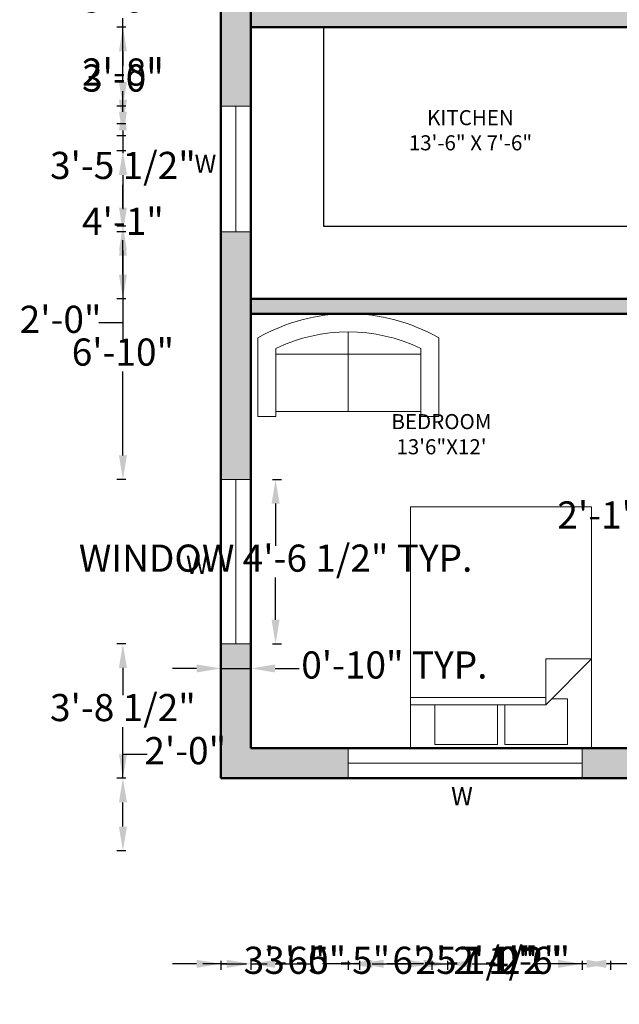
# Model space of a CAD drawing. Units: inches. Extents: x 2568 to 3190, y 746 to 1467.
# Tile 1 of 7: x 2568 to 2767, y 746 to 1073. Entities that reach past the tile are written whole.
import ezdxf

# ---------------------------------------------------------------- set-up
doc = ezdxf.new("R2010")
doc.units = ezdxf.units.IN
for name, color, linetype, lineweight in [('A-ANNO-DIMS', 2, 'Continuous', 18), ('A-ANNO-TEXT', 7, 'Continuous', 18), ('A-AREA-IDEN', 7, 'Continuous', 25), ('A-FLOR-CASE', 8, 'Continuous', 25), ('A-FURN', 8, 'Continuous', 18), ('A-GLAZ', 4, 'Continuous', 20), ('A-WALL', 7, 'Continuous', 50), ('A-WALL-PATT', 252, 'Continuous', 13)]:
    doc.layers.add(name, color=color, linetype=linetype, lineweight=lineweight)
doc.styles.get("Standard").update_dxf_attribs({"font": 'arial.ttf'})
doc.dimstyles.new('ISO-25', dxfattribs={"dimtxt": 9, "dimasz": 8, "dimexe": 2, "dimexo": 1, "dimtad": 0, "dimtih": 1, "dimtoh": 1, "dimdec": 1, "dimlunit": 3, "dimtxsty": 'Standard', "dimcen": 2.5, "dimclrd": 1, "dimclre": 3, "dimclrt": 6, "dimadec": 0, "dimazin": 0, "dimtfac": 1, "dimtdec": 1, "dimtmove": 0, "dimatfit": 3, "dimfxl": 1, "dimfxlon": 1, "dimarcsym": 0})

# ---------------------------------------------------------------- blocks, each defined once
blk = doc.blocks.new('Bed - Queen')
for p, q in [((0, -80.00003), (0, 0)), ((0, 0), (59.99999, 0)), ((59.99999, 0), (59.99999, -80.00003)), ((7.99999, -1.2), (28.79998, -1.2)), ((7.99999, -14.4), (7.99999, -1.2)), ((28.79998, -1.2), (28.79998, -14.4)), ((31.19999, -1.2), (51.99999, -1.2)), ((31.19999, -14.4), (31.19999, -1.2)), ((51.99999, -1.2), (51.99999, -16.4)), ((0, -14.4), (44.8, -14.4)), ((59.99999, -29.6), (44.8, -14.4)), ((44.8, -14.4), (44.8, -29.6)), ((44.8, -16.8), (0, -16.8)), ((51.99999, -16.4), (46.79936, -16.4)), ((44.8, -29.6), (59.99999, -29.6)), ((59.99999, -80.00003), (0, -80.00003))]:
    blk.add_line(p, q)
blk = doc.blocks.new('Sofa - Roundback Loveseat 5 ft.')
for p, q in [((0, -32.44198), (0, -5.99998)), ((-24, -33.99998), (-24, -11.46958)), ((24.00004, -33.99998), (24.00004, -11.46958)), ((-23.9998, -13.38178), (23.99986, -13.38178)), ((-24, -32.44198), (24.00004, -32.44198))]:
    blk.add_line(p, q)
for points in [[(-24, -33.99998), (-30, -33.99998), (-30, -7.99998)], [(30.00004, -7.99998), (30.00004, -33.99998), (24.00004, -33.99998)]]:
    blk.add_lwpolyline(points)
for centre, radius, start, end in [((0, -60.24998), 60.24998, 60.13715, 119.8628), ((0, -61.38438), 55.38444, 64.32083, 115.6792)]:
    blk.add_arc(centre, radius, start, end)
blk = doc.blocks.new('WIN-BED-LOWER-54.48')
for p, q in [((-5, 54.48), (5, 54.48)), ((0, 0), (0, 54.48)), ((5, 0), (-5, 0))]:
    blk.add_line(p, q)
blk = doc.blocks.new('*D26')
at = {"layer": 'A-ANNO-DIMS', "color": 1, "lineweight": -2, "transparency": 16777216}
for p, q in [((2809.71, 907.49), (2801.71, 907.49)), ((2826.58, 907.49), (2817.71, 907.49))]:
    blk.add_line(p, q, dxfattribs=at)
at = {"layer": 'A-ANNO-DIMS', "color": 3, "lineweight": -2, "transparency": 16777216}
for p, q in [((2809.71, 906.49), (2809.71, 909.49)), ((2834.58, 906.49), (2834.58, 909.49))]:
    blk.add_line(p, q, dxfattribs=at)
at = {"layer": 'A-ANNO-DIMS', "color": 1, "transparency": 16777216}
for points in [[(2817.71, 908.82), (2817.71, 906.15), (2809.71, 907.49)], [(2826.58, 908.82), (2826.58, 906.15), (2834.58, 907.49)]]:
    blk.add_solid(points, dxfattribs=at)
at = {"layer": 'Defpoints', "color": 0, "transparency": 16777216}
for p in [(2809.71, 907.49), (2809.71, 898.94), (2834.58, 898.94)]:
    blk.add_point(p, dxfattribs=at)
at = {"layer": 'A-ANNO-DIMS', "color": 6, "transparency": 16777216, "insert": (2773.58, 907.49), "char_height": 9, "attachment_point": 5}
blk.add_mtext('2\'-1" TYP.', dxfattribs=at)
blk = doc.blocks.new('*D35')
at = {"layer": 'A-ANNO-DIMS', "color": 3, "lineweight": -2, "transparency": 16777216}
for p, q in [((2651.69, 920.42), (2654.69, 920.42)), ((2651.69, 865.93), (2654.69, 865.93))]:
    blk.add_line(p, q, dxfattribs=at)
at = {"layer": 'A-ANNO-DIMS', "color": 1, "lineweight": -2, "transparency": 16777216}
for p, q in [((2652.69, 912.42), (2652.69, 898.46)), ((2652.69, 873.93), (2652.69, 887.89))]:
    blk.add_line(p, q, dxfattribs=at)
at = {"layer": 'A-ANNO-DIMS', "color": 1, "transparency": 16777216}
for points in [[(2651.36, 912.42), (2654.03, 912.42), (2652.69, 920.42)], [(2651.36, 873.93), (2654.03, 873.93), (2652.69, 865.93)]]:
    blk.add_solid(points, dxfattribs=at)
at = {"layer": 'Defpoints', "color": 0, "transparency": 16777216}
for p in [(2644.52, 920.42), (2652.69, 920.42), (2644.52, 865.93)]:
    blk.add_point(p, dxfattribs=at)
at = {"layer": 'A-ANNO-DIMS', "color": 6, "transparency": 16777216, "insert": (2652.69, 893.17), "char_height": 9, "attachment_point": 5}
blk.add_mtext('WINDOW 4\'-6 1/2" TYP.', dxfattribs=at)
blk = doc.blocks.new('*D36')
at = {"layer": 'A-ANNO-DIMS', "color": 3, "lineweight": -2, "transparency": 16777216}
for p, q in [((2634.52, 858.76), (2634.52, 855.76)), ((2644.52, 858.76), (2644.52, 855.76))]:
    blk.add_line(p, q, dxfattribs=at)
at = {"layer": 'A-ANNO-DIMS', "color": 1, "lineweight": -2, "transparency": 16777216}
for p, q in [((2626.52, 857.76), (2618.52, 857.76)), ((2634.52, 857.76), (2644.52, 857.76)), ((2652.52, 857.76), (2660.52, 857.76))]:
    blk.add_line(p, q, dxfattribs=at)
at = {"layer": 'A-ANNO-DIMS', "color": 1, "transparency": 16777216}
for points in [[(2626.52, 859.1), (2626.52, 856.43), (2634.52, 857.76)], [(2652.52, 859.1), (2652.52, 856.43), (2644.52, 857.76)]]:
    blk.add_solid(points, dxfattribs=at)
at = {"layer": 'Defpoints', "color": 0, "transparency": 16777216}
for p in [(2634.52, 865.93), (2644.52, 865.93), (2644.52, 857.76)]:
    blk.add_point(p, dxfattribs=at)
at = {"layer": 'A-ANNO-DIMS', "color": 6, "transparency": 16777216, "insert": (2692.07, 857.76), "char_height": 9, "attachment_point": 5}
blk.add_mtext('0\'-10" TYP.', dxfattribs=at)
blk = doc.blocks.new('*D39')
at = {"layer": 'A-ANNO-DIMS', "color": 3, "lineweight": -2, "transparency": 16777216}
for p, q in [((2644.52, 760.85), (2644.52, 757.85)), ((2709.74, 760.85), (2709.74, 757.85))]:
    blk.add_line(p, q, dxfattribs=at)
at = {"layer": 'A-ANNO-DIMS', "color": 1, "lineweight": -2, "transparency": 16777216}
for p, q in [((2652.52, 759.85), (2664.54, 759.85)), ((2701.74, 759.85), (2689.72, 759.85))]:
    blk.add_line(p, q, dxfattribs=at)
at = {"layer": 'A-ANNO-DIMS', "color": 1, "transparency": 16777216}
for points in [[(2652.52, 761.18), (2652.52, 758.51), (2644.52, 759.85)], [(2701.74, 761.18), (2701.74, 758.51), (2709.74, 759.85)]]:
    blk.add_solid(points, dxfattribs=at)
at = {"layer": 'Defpoints', "color": 0, "transparency": 16777216}
for p in [(2644.52, 1411.35), (2709.74, 1411.35), (2709.74, 759.85)]:
    blk.add_point(p, dxfattribs=at)
at = {"layer": 'A-ANNO-DIMS', "color": 6, "transparency": 16777216, "insert": (2677.13, 759.85), "char_height": 9, "attachment_point": 5}
blk.add_mtext('5\'-5"', dxfattribs=at)
blk = doc.blocks.new('*D40')
at = {"layer": 'A-ANNO-DIMS', "color": 3, "lineweight": -2, "transparency": 16777216}
for p, q in [((2709.74, 760.85), (2709.74, 757.85)), ((2763.78, 760.85), (2763.78, 757.85))]:
    blk.add_line(p, q, dxfattribs=at)
at = {"layer": 'A-ANNO-DIMS', "color": 1, "lineweight": -2, "transparency": 16777216}
for p, q in [((2717.74, 759.85), (2723.99, 759.85)), ((2755.78, 759.85), (2749.52, 759.85))]:
    blk.add_line(p, q, dxfattribs=at)
at = {"layer": 'A-ANNO-DIMS', "color": 1, "transparency": 16777216}
for points in [[(2717.74, 761.18), (2717.74, 758.51), (2709.74, 759.85)], [(2755.78, 761.18), (2755.78, 758.51), (2763.78, 759.85)]]:
    blk.add_solid(points, dxfattribs=at)
at = {"layer": 'Defpoints', "color": 0, "transparency": 16777216}
for p in [(2709.74, 1411.35), (2763.78, 1411.35), (2763.78, 759.85)]:
    blk.add_point(p, dxfattribs=at)
at = {"layer": 'A-ANNO-DIMS', "color": 6, "transparency": 16777216, "insert": (2736.76, 759.85), "char_height": 9, "attachment_point": 5}
blk.add_mtext('4\'-6"', dxfattribs=at)
blk = doc.blocks.new('*D45')
at = {"layer": 'A-ANNO-DIMS', "color": 3, "lineweight": -2, "transparency": 16777216}
for p, q in [((2634.52, 760.85), (2634.52, 757.85)), ((2676.76, 760.85), (2676.76, 757.85))]:
    blk.add_line(p, q, dxfattribs=at)
at = {"layer": 'A-ANNO-DIMS', "color": 1, "lineweight": -2, "transparency": 16777216}
for p, q in [((2626.52, 759.85), (2618.52, 759.85)), ((2634.52, 759.85), (2643.06, 759.85)), ((2676.76, 759.85), (2668.23, 759.85)), ((2684.76, 759.85), (2692.76, 759.85))]:
    blk.add_line(p, q, dxfattribs=at)
at = {"layer": 'A-ANNO-DIMS', "color": 1, "transparency": 16777216}
for points in [[(2626.52, 761.18), (2626.52, 758.51), (2634.52, 759.85)], [(2684.76, 761.18), (2684.76, 758.51), (2676.76, 759.85)]]:
    blk.add_solid(points, dxfattribs=at)
at = {"layer": 'Defpoints', "color": 0, "transparency": 16777216}
for p in [(2634.52, 821.35), (2676.76, 821.35), (2676.76, 759.85)]:
    blk.add_point(p, dxfattribs=at)
at = {"layer": 'A-ANNO-DIMS', "color": 6, "transparency": 16777216, "insert": (2655.64, 759.85), "char_height": 9, "attachment_point": 5}
blk.add_mtext('3\'-6"', dxfattribs=at)
blk = doc.blocks.new('*D46')
at = {"layer": 'A-ANNO-DIMS', "color": 3, "lineweight": -2, "transparency": 16777216}
for p, q in [((2676.76, 760.85), (2676.76, 757.85)), ((2754.37, 760.85), (2754.37, 757.85))]:
    blk.add_line(p, q, dxfattribs=at)
at = {"layer": 'A-ANNO-DIMS', "color": 1, "lineweight": -2, "transparency": 16777216}
for p, q in [((2684.76, 759.85), (2692.47, 759.85)), ((2746.37, 759.85), (2738.66, 759.85))]:
    blk.add_line(p, q, dxfattribs=at)
at = {"layer": 'A-ANNO-DIMS', "color": 1, "transparency": 16777216}
for points in [[(2684.76, 761.18), (2684.76, 758.51), (2676.76, 759.85)], [(2746.37, 761.18), (2746.37, 758.51), (2754.37, 759.85)]]:
    blk.add_solid(points, dxfattribs=at)
at = {"layer": 'Defpoints', "color": 0, "transparency": 16777216}
for p in [(2676.76, 821.35), (2754.37, 821.35), (2754.37, 759.85)]:
    blk.add_point(p, dxfattribs=at)
at = {"layer": 'A-ANNO-DIMS', "color": 6, "transparency": 16777216, "insert": (2715.56, 759.85), "char_height": 9, "attachment_point": 5}
blk.add_mtext('6\'-5 1/2"', dxfattribs=at)
blk = doc.blocks.new('*D47')
at = {"layer": 'A-ANNO-DIMS', "color": 3, "lineweight": -2, "transparency": 16777216}
for p, q in [((2754.37, 1452.8), (2754.37, 1455.8)), ((2846.86, 1452.8), (2846.86, 1455.8))]:
    blk.add_line(p, q, dxfattribs=at)
at = {"layer": 'A-ANNO-DIMS', "color": 1, "lineweight": -2, "transparency": 16777216}
for p, q in [((2762.37, 1453.8), (2777.58, 1453.8)), ((2838.86, 1453.8), (2823.65, 1453.8))]:
    blk.add_line(p, q, dxfattribs=at)
at = {"layer": 'A-ANNO-DIMS', "color": 1, "transparency": 16777216}
for points in [[(2762.37, 1455.13), (2762.37, 1452.47), (2754.37, 1453.8)], [(2838.86, 1455.13), (2838.86, 1452.47), (2846.86, 1453.8)]]:
    blk.add_solid(points, dxfattribs=at)
at = {"layer": 'Defpoints', "color": 0, "transparency": 16777216}
for p in [(2846.86, 1453.8), (2754.37, 831.35), (2846.86, 831.35)]:
    blk.add_point(p, dxfattribs=at)
at = {"layer": 'A-ANNO-DIMS', "color": 6, "transparency": 16777216, "insert": (2800.61, 1453.8), "char_height": 9, "attachment_point": 5}
blk.add_mtext('7\'-8 1/2"', dxfattribs=at)
blk = doc.blocks.new('*D52')
at = {"layer": 'A-ANNO-DIMS', "color": 1, "lineweight": -2, "transparency": 16777216}
for p, q in [((2602.07, 821.35), (2602.07, 829.35)), ((2602.07, 829.35), (2610.07, 829.35)), ((2602.07, 805.35), (2602.07, 813.35))]:
    blk.add_line(p, q, dxfattribs=at)
at = {"layer": 'A-ANNO-DIMS', "color": 3, "lineweight": -2, "transparency": 16777216}
for p, q in [((2603.07, 821.35), (2600.07, 821.35)), ((2603.07, 797.35), (2600.07, 797.35))]:
    blk.add_line(p, q, dxfattribs=at)
at = {"layer": 'A-ANNO-DIMS', "color": 1, "transparency": 16777216}
for points in [[(2600.74, 813.35), (2603.41, 813.35), (2602.07, 821.35)], [(2600.74, 805.35), (2603.41, 805.35), (2602.07, 797.35)]]:
    blk.add_solid(points, dxfattribs=at)
at = {"layer": 'Defpoints', "color": 0, "transparency": 16777216}
for p in [(2602.07, 821.35), (2785.87, 821.35), (2785.87, 797.35)]:
    blk.add_point(p, dxfattribs=at)
at = {"layer": 'A-ANNO-DIMS', "color": 6, "transparency": 16777216, "insert": (2622.74, 829.35), "char_height": 9, "attachment_point": 5}
blk.add_mtext('2\'-0"', dxfattribs=at)
blk = doc.blocks.new('*D56')
at = {"layer": 'A-ANNO-DIMS', "color": 3, "lineweight": -2, "transparency": 16777216}
for p, q in [((2603.07, 1070.35), (2600.07, 1070.35)), ((2603.07, 1034.35), (2600.07, 1034.35))]:
    blk.add_line(p, q, dxfattribs=at)
at = {"layer": 'A-ANNO-DIMS', "color": 1, "lineweight": -2, "transparency": 16777216}
for p, q in [((2602.07, 1062.35), (2602.07, 1057.57)), ((2602.07, 1042.35), (2602.07, 1047.13))]:
    blk.add_line(p, q, dxfattribs=at)
at = {"layer": 'A-ANNO-DIMS', "color": 1, "transparency": 16777216}
for points in [[(2600.74, 1062.35), (2603.41, 1062.35), (2602.07, 1070.35)], [(2600.74, 1042.35), (2603.41, 1042.35), (2602.07, 1034.35)]]:
    blk.add_solid(points, dxfattribs=at)
at = {"layer": 'Defpoints', "color": 0, "transparency": 16777216}
for p in [(2602.07, 1070.35), (2974.52, 1070.35), (2974.52, 1034.35)]:
    blk.add_point(p, dxfattribs=at)
at = {"layer": 'A-ANNO-DIMS', "color": 6, "transparency": 16777216, "insert": (2602.07, 1052.35), "char_height": 9, "attachment_point": 5}
blk.add_mtext('3\'-0"', dxfattribs=at)
blk = doc.blocks.new('*D58')
at = {"layer": 'A-ANNO-DIMS', "color": 3, "lineweight": -2, "transparency": 16777216}
for p, q in [((2603.07, 1029.35), (2600.07, 1029.35)), ((2603.07, 980.35), (2600.07, 980.35))]:
    blk.add_line(p, q, dxfattribs=at)
at = {"layer": 'A-ANNO-DIMS', "color": 1, "lineweight": -2, "transparency": 16777216}
for p, q in [((2602.07, 1021.35), (2602.07, 1009.99)), ((2602.07, 988.35), (2602.07, 999.71))]:
    blk.add_line(p, q, dxfattribs=at)
at = {"layer": 'A-ANNO-DIMS', "color": 1, "transparency": 16777216}
for points in [[(2600.74, 1021.35), (2603.41, 1021.35), (2602.07, 1029.35)], [(2600.74, 988.35), (2603.41, 988.35), (2602.07, 980.35)]]:
    blk.add_solid(points, dxfattribs=at)
at = {"layer": 'Defpoints', "color": 0, "transparency": 16777216}
for p in [(3044.52, 1029.35), (2602.07, 980.35), (3043.77, 980.35)]:
    blk.add_point(p, dxfattribs=at)
at = {"layer": 'A-ANNO-DIMS', "color": 6, "transparency": 16777216, "insert": (2602.07, 1004.85), "char_height": 9, "attachment_point": 5}
blk.add_mtext('4\'-1"', dxfattribs=at)
blk = doc.blocks.new('*D62')
at = {"layer": 'A-ANNO-DIMS', "color": 3, "lineweight": -2, "transparency": 16777216}
for p, q in [((2603.07, 1004.35), (2600.07, 1004.35)), ((2603.07, 980.35), (2600.07, 980.35))]:
    blk.add_line(p, q, dxfattribs=at)
at = {"layer": 'A-ANNO-DIMS', "color": 1, "lineweight": -2, "transparency": 16777216}
for p, q in [((2602.07, 996.35), (2602.07, 988.35)), ((2602.07, 980.35), (2602.07, 972.35)), ((2602.07, 972.35), (2594.07, 972.35))]:
    blk.add_line(p, q, dxfattribs=at)
at = {"layer": 'A-ANNO-DIMS', "color": 1, "transparency": 16777216}
for points in [[(2600.74, 996.35), (2603.41, 996.35), (2602.07, 1004.35)], [(2600.74, 988.35), (2603.41, 988.35), (2602.07, 980.35)]]:
    blk.add_solid(points, dxfattribs=at)
at = {"layer": 'Defpoints', "color": 0, "transparency": 16777216}
for p in [(3044.52, 1004.35), (2602.07, 980.35), (3043.77, 980.35)]:
    blk.add_point(p, dxfattribs=at)
at = {"layer": 'A-ANNO-DIMS', "color": 6, "transparency": 16777216, "insert": (2581.41, 972.35), "char_height": 9, "attachment_point": 5}
blk.add_mtext('2\'-0"', dxfattribs=at)
blk = doc.blocks.new('*D64')
at = {"layer": 'A-ANNO-DIMS', "color": 3, "lineweight": -2, "transparency": 16777216}
for p, q in [((2644.52, 760.85), (2644.52, 757.85)), ((2680.52, 760.85), (2680.52, 757.85))]:
    blk.add_line(p, q, dxfattribs=at)
at = {"layer": 'A-ANNO-DIMS', "color": 1, "lineweight": -2, "transparency": 16777216}
for p, q in [((2636.52, 759.85), (2628.52, 759.85)), ((2644.52, 759.85), (2649.94, 759.85)), ((2680.52, 759.85), (2675.11, 759.85)), ((2688.52, 759.85), (2696.52, 759.85))]:
    blk.add_line(p, q, dxfattribs=at)
at = {"layer": 'A-ANNO-DIMS', "color": 1, "transparency": 16777216}
for points in [[(2636.52, 761.18), (2636.52, 758.51), (2644.52, 759.85)], [(2688.52, 761.18), (2688.52, 758.51), (2680.52, 759.85)]]:
    blk.add_solid(points, dxfattribs=at)
at = {"layer": 'Defpoints', "color": 0, "transparency": 16777216}
for p in [(2644.52, 1261.35), (2680.52, 1262.35), (2680.52, 759.85)]:
    blk.add_point(p, dxfattribs=at)
at = {"layer": 'A-ANNO-DIMS', "color": 6, "transparency": 16777216, "insert": (2662.52, 759.85), "char_height": 9, "attachment_point": 5}
blk.add_mtext('3\'-0"', dxfattribs=at)
blk = doc.blocks.new('*D65')
at = {"layer": 'A-ANNO-DIMS', "color": 3, "lineweight": -2, "transparency": 16777216}
for p, q in [((2680.52, 760.85), (2680.52, 757.85)), ((2704.52, 760.85), (2704.52, 757.85))]:
    blk.add_line(p, q, dxfattribs=at)
at = {"layer": 'A-ANNO-DIMS', "color": 1, "lineweight": -2, "transparency": 16777216}
for p, q in [((2688.52, 759.85), (2696.52, 759.85)), ((2704.52, 759.85), (2712.52, 759.85))]:
    blk.add_line(p, q, dxfattribs=at)
at = {"layer": 'A-ANNO-DIMS', "color": 1, "transparency": 16777216}
for points in [[(2688.52, 761.18), (2688.52, 758.51), (2680.52, 759.85)], [(2696.52, 761.18), (2696.52, 758.51), (2704.52, 759.85)]]:
    blk.add_solid(points, dxfattribs=at)
at = {"layer": 'Defpoints', "color": 0, "transparency": 16777216}
for p in [(2680.52, 1262.35), (2704.52, 1261.35), (2704.52, 759.85)]:
    blk.add_point(p, dxfattribs=at)
at = {"layer": 'A-ANNO-DIMS', "color": 6, "transparency": 16777216, "insert": (2725.19, 759.85), "char_height": 9, "attachment_point": 5}
blk.add_mtext('2\'-0"', dxfattribs=at)
blk = doc.blocks.new('*D66')
at = {"layer": 'A-ANNO-DIMS', "color": 3, "lineweight": -2, "transparency": 16777216}
for p, q in [((2603.07, 865.93), (2600.07, 865.93)), ((2603.07, 821.35), (2600.07, 821.35))]:
    blk.add_line(p, q, dxfattribs=at)
at = {"layer": 'A-ANNO-DIMS', "color": 1, "lineweight": -2, "transparency": 16777216}
for p, q in [((2602.07, 857.93), (2602.07, 848.92)), ((2602.07, 829.35), (2602.07, 838.36))]:
    blk.add_line(p, q, dxfattribs=at)
at = {"layer": 'A-ANNO-DIMS', "color": 1, "transparency": 16777216}
for points in [[(2600.74, 857.93), (2603.41, 857.93), (2602.07, 865.93)], [(2600.74, 829.35), (2603.41, 829.35), (2602.07, 821.35)]]:
    blk.add_solid(points, dxfattribs=at)
at = {"layer": 'Defpoints', "color": 0, "transparency": 16777216}
for p in [(2602.07, 865.93), (2634.52, 865.93), (2634.52, 821.35)]:
    blk.add_point(p, dxfattribs=at)
at = {"layer": 'A-ANNO-DIMS', "color": 6, "transparency": 16777216, "insert": (2602.07, 843.64), "char_height": 9, "attachment_point": 5}
blk.add_mtext('3\'-8 1/2"', dxfattribs=at)
blk = doc.blocks.new('*D67')
at = {"layer": 'A-ANNO-DIMS', "color": 3, "lineweight": -2, "transparency": 16777216}
for p, q in [((2603.07, 1002.57), (2600.07, 1002.57)), ((2603.07, 920.42), (2600.07, 920.42))]:
    blk.add_line(p, q, dxfattribs=at)
at = {"layer": 'A-ANNO-DIMS', "color": 1, "lineweight": -2, "transparency": 16777216}
for p, q in [((2602.07, 994.57), (2602.07, 966.71)), ((2602.07, 928.42), (2602.07, 956.27))]:
    blk.add_line(p, q, dxfattribs=at)
at = {"layer": 'A-ANNO-DIMS', "color": 1, "transparency": 16777216}
for points in [[(2600.74, 994.57), (2603.41, 994.57), (2602.07, 1002.57)], [(2600.74, 928.42), (2603.41, 928.42), (2602.07, 920.42)]]:
    blk.add_solid(points, dxfattribs=at)
at = {"layer": 'Defpoints', "color": 0, "transparency": 16777216}
for p in [(2602.07, 1002.57), (2634.52, 1002.57), (2634.52, 920.42)]:
    blk.add_point(p, dxfattribs=at)
at = {"layer": 'A-ANNO-DIMS', "color": 6, "transparency": 16777216, "insert": (2602.07, 961.49), "char_height": 9, "attachment_point": 5}
blk.add_mtext('6\'-10"', dxfattribs=at)
blk = doc.blocks.new('*D68')
at = {"layer": 'A-ANNO-DIMS', "color": 3, "lineweight": -2, "transparency": 16777216}
for p, q in [((2603.07, 1044.16), (2600.07, 1044.16)), ((2603.07, 1002.57), (2600.07, 1002.57))]:
    blk.add_line(p, q, dxfattribs=at)
at = {"layer": 'A-ANNO-DIMS', "color": 1, "lineweight": -2, "transparency": 16777216}
for p, q in [((2602.07, 1036.16), (2602.07, 1028.65)), ((2602.07, 1010.57), (2602.07, 1018.09))]:
    blk.add_line(p, q, dxfattribs=at)
at = {"layer": 'A-ANNO-DIMS', "color": 1, "transparency": 16777216}
for points in [[(2600.74, 1036.16), (2603.41, 1036.16), (2602.07, 1044.16)], [(2600.74, 1010.57), (2603.41, 1010.57), (2602.07, 1002.57)]]:
    blk.add_solid(points, dxfattribs=at)
at = {"layer": 'Defpoints', "color": 0, "transparency": 16777216}
for p in [(2602.07, 1044.16), (2634.52, 1044.16), (2634.52, 1002.57)]:
    blk.add_point(p, dxfattribs=at)
at = {"layer": 'A-ANNO-DIMS', "color": 6, "transparency": 16777216, "insert": (2602.07, 1023.37), "char_height": 9, "attachment_point": 5}
blk.add_mtext('3\'-5 1/2"', dxfattribs=at)
blk = doc.blocks.new('*D69')
at = {"layer": 'A-ANNO-DIMS', "color": 3, "lineweight": -2, "transparency": 16777216}
for p, q in [((2603.07, 1113), (2600.07, 1113)), ((2603.07, 1044.16), (2600.07, 1044.16))]:
    blk.add_line(p, q, dxfattribs=at)
at = {"layer": 'A-ANNO-DIMS', "color": 1, "lineweight": -2, "transparency": 16777216}
for p, q in [((2602.07, 1105), (2602.07, 1083.8)), ((2602.07, 1052.16), (2602.07, 1073.36))]:
    blk.add_line(p, q, dxfattribs=at)
at = {"layer": 'A-ANNO-DIMS', "color": 1, "transparency": 16777216}
for points in [[(2600.74, 1105), (2603.41, 1105), (2602.07, 1113)], [(2600.74, 1052.16), (2603.41, 1052.16), (2602.07, 1044.16)]]:
    blk.add_solid(points, dxfattribs=at)
at = {"layer": 'Defpoints', "color": 0, "transparency": 16777216}
for p in [(2602.07, 1113), (2634.52, 1113), (2634.52, 1044.16)]:
    blk.add_point(p, dxfattribs=at)
at = {"layer": 'A-ANNO-DIMS', "color": 6, "transparency": 16777216, "insert": (2602.07, 1078.58), "char_height": 9, "attachment_point": 5}
blk.add_mtext('5\'-9"', dxfattribs=at)
blk = doc.blocks.new('*D74')
at = {"layer": 'A-ANNO-DIMS', "color": 3, "lineweight": -2, "transparency": 16777216}
for p, q in [((2603.07, 1070.35), (2600.07, 1070.35)), ((2603.07, 1038.35), (2600.07, 1038.35))]:
    blk.add_line(p, q, dxfattribs=at)
at = {"layer": 'A-ANNO-DIMS', "color": 1, "lineweight": -2, "transparency": 16777216}
for p, q in [((2602.07, 1062.35), (2602.07, 1059.57)), ((2602.07, 1046.35), (2602.07, 1049.13))]:
    blk.add_line(p, q, dxfattribs=at)
at = {"layer": 'A-ANNO-DIMS', "color": 1, "transparency": 16777216}
for points in [[(2600.74, 1062.35), (2603.41, 1062.35), (2602.07, 1070.35)], [(2600.74, 1046.35), (2603.41, 1046.35), (2602.07, 1038.35)]]:
    blk.add_solid(points, dxfattribs=at)
at = {"layer": 'Defpoints', "color": 0, "transparency": 16777216}
for p in [(2602.07, 1070.35), (2806.52, 1070.35), (2806.52, 1038.35)]:
    blk.add_point(p, dxfattribs=at)
at = {"layer": 'A-ANNO-DIMS', "color": 6, "transparency": 16777216, "insert": (2602.07, 1054.35), "char_height": 9, "attachment_point": 5}
blk.add_mtext('2\'-8"', dxfattribs=at)
blk = doc.blocks.new('*D83')
at = {"layer": 'A-ANNO-DIMS', "color": 3, "lineweight": -2, "transparency": 16777216}
for p, q in [((2754.37, 760.85), (2754.37, 757.85)), ((2785.87, 760.85), (2785.87, 757.85))]:
    blk.add_line(p, q, dxfattribs=at)
at = {"layer": 'A-ANNO-DIMS', "color": 1, "lineweight": -2, "transparency": 16777216}
for p, q in [((2754.37, 759.85), (2746.37, 759.85)), ((2777.87, 759.85), (2762.37, 759.85))]:
    blk.add_line(p, q, dxfattribs=at)
at = {"layer": 'A-ANNO-DIMS', "color": 1, "transparency": 16777216}
for points in [[(2762.37, 761.18), (2762.37, 758.51), (2754.37, 759.85)], [(2777.87, 761.18), (2777.87, 758.51), (2785.87, 759.85)]]:
    blk.add_solid(points, dxfattribs=at)
at = {"layer": 'Defpoints', "color": 0, "transparency": 16777216}
for p in [(2754.37, 821.35), (2785.87, 797.35), (2754.37, 759.85)]:
    blk.add_point(p, dxfattribs=at)
at = {"layer": 'A-ANNO-DIMS', "color": 6, "transparency": 16777216, "insert": (2723.22, 759.85), "char_height": 9, "attachment_point": 5}
blk.add_mtext('2\'-7 1/2"', dxfattribs=at)

msp = doc.modelspace()

# ---------------------------------------------------------------- hatches: boundary and pattern name
at = {"layer": 'A-WALL-PATT'}
h = msp.add_hatch(color=256, dxfattribs=at)
h.dxf.hatch_style = 1
h.paths.add_polyline_path([(2709.74, 1411.35), (2709.74, 1421.35), (2634.52, 1421.35), (2634.52, 1371.08), (2644.52, 1371.08), (2644.52, 1411.35)])
h.paths.add_polyline_path([(2844.66, 1411.35), (2844.66, 1421.35), (2763.78, 1421.35), (2763.78, 1411.35)])
h.paths.add_polyline_path([(2996.2, 1411.35), (2996.2, 1421.35), (2897.43, 1421.35), (2897.43, 1411.35)])
h.paths.add_polyline_path([(3104.52, 1411.35), (3104.52, 1371.08), (3114.52, 1371.08), (3114.52, 1421.35), (3052.64, 1421.35), (3052.64, 1411.35)])
h.paths.add_polyline_path([(3114.52, 1316.62), (3104.52, 1316.62), (3104.52, 1248.37), (3114.52, 1248.37)])
h.paths.add_polyline_path([(3104.52, 1174.04), (3114.52, 1174.04), (3114.52, 1222.08), (3104.52, 1222.08)])
h.paths.add_polyline_path([(3104.52, 1020.11), (3114.52, 1020.11), (3114.52, 1113), (3104.52, 1113)])
h.paths.add_polyline_path([(3104.52, 920.42), (3114.52, 920.42), (3114.52, 992.96), (3104.52, 992.96)])
h.paths.add_polyline_path([(3114.52, 821.35), (3114.52, 865.93), (3104.52, 865.93), (3104.52, 831.35), (3055.78, 831.35), (3055.78, 821.35)])
h.paths.add_polyline_path([(2902.21, 831.35), (2902.21, 821.35), (2986.63, 821.35), (2986.63, 831.35)])
h.paths.add_polyline_path([(2634.52, 821.35), (2676.76, 821.35), (2676.76, 831.35), (2644.52, 831.35), (2644.52, 865.93), (2634.52, 865.93)])
h.paths.add_polyline_path([(2754.37, 821.35), (2846.86, 821.35), (2846.86, 831.35), (2754.37, 831.35)])
h.paths.add_polyline_path([(2644.52, 920.42), (2644.52, 1002.57), (2634.52, 1002.57), (2634.52, 920.42)])
h.paths.add_polyline_path([(2644.52, 1044.16), (2644.52, 1113), (2634.52, 1113), (2634.52, 1044.16)])
h.paths.add_polyline_path([(2644.52, 1248.37), (2644.52, 1316.62), (2634.52, 1316.62), (2634.52, 1248.37)])
h.paths.add_polyline_path([(2634.52, 1222.08), (2634.52, 1174.04), (2644.52, 1174.04), (2644.52, 1222.08)])
h = msp.add_hatch(color=256, dxfattribs=at)
h.dxf.hatch_style = 1
h.paths.add_polyline_path([(2811.52, 1411.35), (2806.52, 1411.35), (2806.52, 1303.35), (2811.52, 1303.35), (2811.52, 1310.35), (2850.52, 1310.35), (2850.52, 1315.35), (2811.52, 1315.35)])
h.paths.add_polyline_path([(2942.52, 1411.35), (2937.52, 1411.35), (2937.52, 1315.35), (2898.52, 1315.35), (2898.52, 1310.35), (2937.52, 1310.35), (2937.52, 1303.35), (2942.52, 1303.35)])
h.paths.add_polyline_path([(2811.52, 1267.35), (2704.52, 1267.35), (2704.52, 1261.35), (2704.52, 1237.35), (2704.52, 1202.35), (2644.52, 1202.35), (2644.52, 1197.35), (2806.52, 1197.35), (2806.52, 1191.38), (2811.52, 1191.38), (2811.52, 1202.35), (2793.52, 1202.35), (2793.52, 1232.35), (2788.52, 1232.35), (2788.52, 1202.35), (2709.52, 1202.35), (2709.52, 1262.35), (2788.52, 1262.35), (2788.52, 1256.35), (2793.52, 1256.35), (2793.52, 1262.35), (2811.52, 1262.35)])
h.paths.add_polyline_path([(2680.52, 1267.35), (2644.52, 1267.35), (2644.52, 1261.35), (2680.52, 1261.35)])
h.paths.add_polyline_path([(3044.52, 1267.35), (2937.52, 1267.35), (2937.52, 1262.35), (2955.52, 1262.35), (2955.52, 1256.35), (2960.52, 1256.35), (2960.52, 1262.35), (3039.52, 1262.35), (3039.52, 1202.35), (2960.52, 1202.35), (2960.52, 1232.35), (2955.52, 1232.35), (2955.52, 1202.35), (2937.52, 1202.35), (2937.52, 1191.38), (2942.52, 1191.38), (2942.52, 1197.35), (3104.52, 1197.35), (3104.52, 1202.35), (3044.52, 1202.35)])
h.paths.add_polyline_path([(3104.52, 1267.35), (3072.52, 1267.35), (3072.52, 1262.35), (3104.52, 1262.35)])
h.paths.add_polyline_path([(2838.1, 1075.35), (2811.52, 1075.35), (2811.52, 1155.35), (2806.52, 1155.35), (2806.52, 1075.35), (2644.52, 1075.35), (2644.52, 1070.35), (2806.52, 1070.35), (2811.52, 1070.35), (2838.1, 1070.35)])
h.paths.add_polyline_path([(3104.52, 1075.35), (2942.52, 1075.35), (2942.52, 1155.38), (2937.52, 1155.38), (2937.52, 1075.35), (2910.92, 1075.35), (2910.92, 1070.35), (2937.52, 1070.35), (3104.52, 1070.35)])
h.paths.add_polyline_path([(2811.52, 1038.35), (2806.52, 1038.35), (2806.52, 980.35), (2644.52, 980.35), (2644.52, 975.35), (2806.52, 975.35), (2806.52, 969.37), (2811.52, 969.37), (2811.52, 975.35)])
h.paths.add_polyline_path([(3104.52, 980.35), (2937.52, 980.35), (2937.52, 969.35), (2942.52, 969.35), (2942.52, 975.35), (3104.52, 975.35)])
h.paths.add_polyline_path([(3104.52, 1034.35), (3039.52, 1034.35), (3039.52, 1004.35), (3044.52, 1004.35), (3044.52, 1029.35), (3104.52, 1029.35)])
h.paths.add_polyline_path([(2942.52, 933.35), (2937.52, 933.35), (2937.52, 831.35), (2942.52, 831.35)])
h.paths.add_polyline_path([(2811.52, 933.37), (2806.52, 933.37), (2806.52, 831.35), (2811.52, 831.35)])

# ---------------------------------------------------------------- linework, layer by layer
at = {"layer": 'A-FLOR-CASE'}
for p, q in [((2668.52, 1070.35), (2668.52, 1004.35)), ((2668.52, 1004.35), (2806.52, 1004.35))]:
    msp.add_line(p, q, dxfattribs=at)
at = {"layer": 'A-GLAZ'}
for p, q in [((2634.52, 1044.16), (2644.52, 1044.16)), ((2639.52, 1002.57), (2639.52, 1044.16)), ((2634.52, 1002.57), (2644.52, 1002.57)), ((2676.76, 831.35), (2676.76, 821.35)), ((2754.37, 831.35), (2754.37, 821.35)), ((2676.76, 826.35), (2754.37, 826.35))]:
    msp.add_line(p, q, dxfattribs=at)
at = {"layer": 'A-WALL'}
for p, q in [((2634.52, 1421.35), (2634.52, 821.35)), ((2644.52, 1411.35), (2644.52, 831.35)), ((2806.52, 1070.35), (2644.52, 1070.35)), ((2806.52, 980.35), (2644.52, 980.35)), ((2806.52, 975.35), (2644.52, 975.35)), ((2644.52, 831.35), (2846.86, 831.35)), ((2634.52, 821.35), (2902.21, 821.35))]:
    msp.add_line(p, q, dxfattribs=at)

# ---------------------------------------------------------------- block references
at = {"layer": 'A-FURN'}
msp.add_blockref('Sofa - Roundback Loveseat 5 ft.', (2676.8, 975.35), dxfattribs=at)
at = {"layer": 'A-FURN', "xscale": -1, "rotation": 180}
msp.add_blockref('Bed - Queen', (2697.47, 831.35), dxfattribs=at)
at = {"layer": 'A-GLAZ'}
msp.add_blockref('WIN-BED-LOWER-54.48', (2639.52, 865.93), dxfattribs=at)

# ---------------------------------------------------------------- texts
at = {"layer": 'A-ANNO-TEXT', "char_height": 6, "attachment_point": 1}
for insert in [(2625.84, 1028.09), (2623.02, 895.11), (2710.89, 818.43)]:
    msp.add_mtext_dynamic_manual_height_columns('W', width=7.7602, gutter_width=12.5, heights=[0], dxfattribs=dict(at, insert=insert))
at = {"layer": 'A-AREA-IDEN', "char_height": 5, "attachment_point": 1}
for s, insert in [('\\pxqc;KITCHEN\\P13\'-6" X 7\'-6"', (2682.36, 1042.87)), ('\\pxqc;BEDROOM\\P13\'6"X12\'', (2672.75, 942.1))]:
    msp.add_mtext_dynamic_manual_height_columns(s, width=69.8646, gutter_width=12.5, heights=[0], dxfattribs=dict(at, insert=insert))

# ---------------------------------------------------------------- dimensions: what is measured, and where the dimension line sits
at = {"layer": 'A-ANNO-DIMS'}
for base, p1, p2, picture, middle in [((2846.86, 1453.8), (2754.37, 831.35), (2846.86, 831.35), '*D47', (2800.61, 1453.8)), ((2709.74, 759.85), (2644.52, 1411.35), (2709.74, 1411.35), '*D39', (2677.13, 759.85)), ((2763.78, 759.85), (2709.74, 1411.35), (2763.78, 1411.35), '*D40', (2736.76, 759.85)), ((2680.52, 759.85), (2644.52, 1261.35), (2680.52, 1262.35), '*D64', (2662.52, 759.85)), ((2704.52, 759.85), (2680.52, 1262.35), (2704.52, 1261.35), '*D65', (2725.19, 759.85)), ((2676.76, 759.85), (2634.52, 821.35), (2676.76, 821.35), '*D45', (2655.64, 759.85)), ((2754.37, 759.85), (2676.76, 821.35), (2754.37, 821.35), '*D46', (2715.56, 759.85)), ((2754.37, 759.85), (2785.87, 797.35), (2754.37, 821.35), '*D83', (2723.22, 759.85))]:
    dim = msp.add_linear_dim(base=base, p1=p1, p2=p2, dimstyle='ISO-25', override={"dimdec": 1, "dimlfac": 1, "dimrnd": 0, "dimzin": 1, "dimdsep": 46, "dimlunit": 4, "dimfrac": 2}, dxfattribs=at)
    dim.commit()
    dim.dimension.update_dxf_attribs({"geometry": picture, "text_midpoint": middle})
for base, p1, p2, picture, middle in [((2602.07, 1113), (2634.52, 1044.16), (2634.52, 1113), '*D69', (2602.07, 1078.58)), ((2602.07, 1070.35), (2974.52, 1034.35), (2974.52, 1070.35), '*D56', (2602.07, 1052.35)), ((2602.07, 1070.35), (2806.52, 1038.35), (2806.52, 1070.35), '*D74', (2602.07, 1054.35)), ((2602.07, 1044.16), (2634.52, 1002.57), (2634.52, 1044.16), '*D68', (2602.07, 1023.37)), ((2602.07, 980.35), (3044.52, 1029.35), (3043.77, 980.35), '*D58', (2602.07, 1004.85)), ((2602.07, 980.35), (3044.52, 1004.35), (3043.77, 980.35), '*D62', (2581.41, 972.35)), ((2602.0725, 1002.5715), (2634.5225, 920.4151), (2634.5225, 1002.5715), '*D67', (2602.0725, 961.4933)), ((2602.07, 865.93), (2634.52, 821.35), (2634.52, 865.93), '*D66', (2602.07, 843.64)), ((2602.07, 821.35), (2785.87, 797.35), (2785.87, 821.35), '*D52', (2622.74, 829.35))]:
    dim = msp.add_linear_dim(base=base, p1=p1, p2=p2, angle=90, dimstyle='ISO-25', override={"dimdec": 1, "dimlfac": 1, "dimrnd": 0, "dimzin": 1, "dimdsep": 46, "dimlunit": 4, "dimfrac": 2}, dxfattribs=at)
    dim.commit()
    dim.dimension.update_dxf_attribs({"geometry": picture, "text_midpoint": middle})
for base, p1, p2, angle, text, picture, middle in [((2652.69, 920.42), (2644.52, 865.93), (2644.52, 920.42), 90, 'WINDOW <> TYP.', '*D35', (2652.69, 893.17)), ((2809.71, 907.49), (2834.58, 898.94), (2809.71, 898.94), 180, '<> TYP.', '*D26', (2773.58, 907.49))]:
    dim = msp.add_linear_dim(base=base, p1=p1, p2=p2, angle=angle, text=text, dimstyle='ISO-25', override={"dimdec": 1, "dimlfac": 1, "dimrnd": 0, "dimzin": 1, "dimdsep": 46, "dimlunit": 4, "dimfrac": 2}, dxfattribs=at)
    dim.commit()
    dim.dimension.update_dxf_attribs({"geometry": picture, "text_midpoint": middle})
dim = msp.add_linear_dim(base=(2644.52, 857.76), p1=(2634.52, 865.93), p2=(2644.52, 865.93), text='<> TYP.', dimstyle='ISO-25', override={"dimdec": 1, "dimlfac": 1, "dimrnd": 0, "dimzin": 1, "dimdsep": 46, "dimlunit": 4, "dimfrac": 2}, dxfattribs=at)
dim.commit()
dim.dimension.update_dxf_attribs({"geometry": '*D36', "text_midpoint": (2692.07, 857.76)})

doc.saveas('drawing.dxf')
